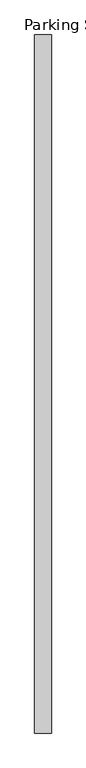
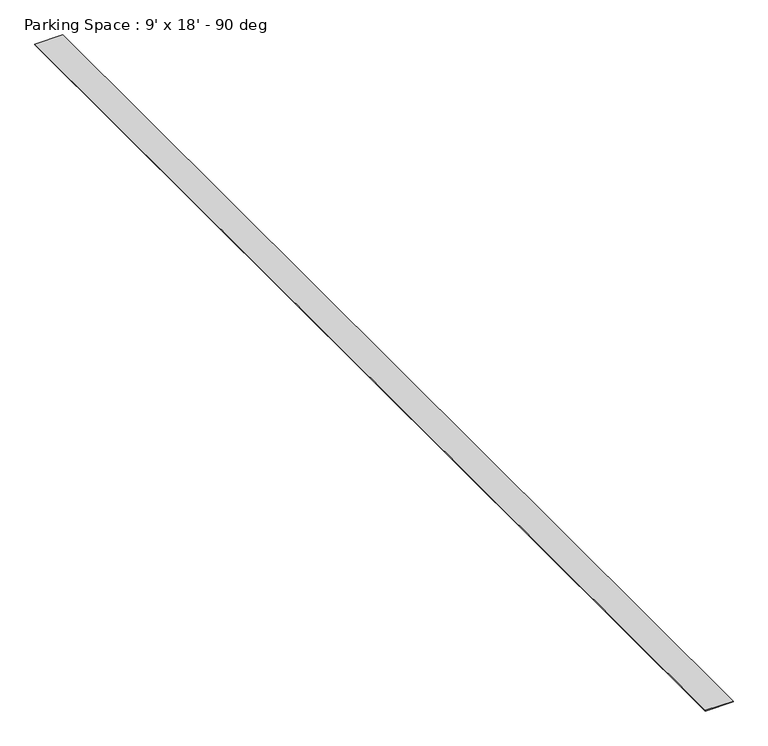
"""IFC4 building model written with IfcOpenShell, lengths in millimetres: proxy geometry, Parking Space : 9' x 18' - 90 deg."""

from ifc_helpers import new_model, si_unit, origin, origin_with_axes, place, context, project, spatial, polyline, outline, extrude, source, transform, mapped, element, save


def parking_space_9_x_18_90_deg_fdd9e8f5(model_context):
    return source(origin(), model_context, "Body", "SweptSolid", [
        extrude(outline(polyline([(-50.8, 0.0), (50.8, 0.0), (50.8, -4267.2), (-50.8, -4267.2), (-50.8, 0.0)])), origin_with_axes(), (0.0, 0.0, 1.0), 3.175),
    ])


if __name__ == "__main__":
    model = new_model("IFC4")
    model_context = context("Model", 3, world=origin())
    ifc_project = project(units=[si_unit("LENGTHUNIT", "METRE", prefix="MILLI")], contexts=[model_context])
    site = spatial("IfcSite", under=ifc_project)
    building = spatial("IfcBuilding", under=site)
    placement = place(None, origin())
    parking_space_9_x_18_90_deg_shape = parking_space_9_x_18_90_deg_fdd9e8f5(model_context)
    element("IfcBuildingElementProxy", 1, Name="Parking Space : 9' x 18' - 90 deg", ObjectType="Parking Space : 9' x 18' - 90 deg", at=placement, inside=building, context=model_context, shape_type="MappedRepresentation", body=[
        mapped(parking_space_9_x_18_90_deg_shape, transform((0.0, 0.0, 0.0), x_axis=(1.0, 0.0, 0.0), y_axis=(0.0, 1.0, 0.0), z_axis=(0.0, 0.0, 1.0))),
    ])
    save(model, "model.ifc")

# Revit data of these elements
# Type "Parking Space : 9' x 18' - 90 deg"
#   Angle = 90.00°
#   Parking Length = 18' - 0"
#   Parking Width = 9' - 0"
#   pl = 14' - 0"
#   pw = 9' - 0"
# Element 1 (IfcBuildingElementProxy, "Parking Space : 9' x 18' - 90 deg")
#   Materials on its faces: "Parking Stripe"
# Materials
#   "Parking Stripe": class "Paint", colour RGB 250 250 91, transparency 0
